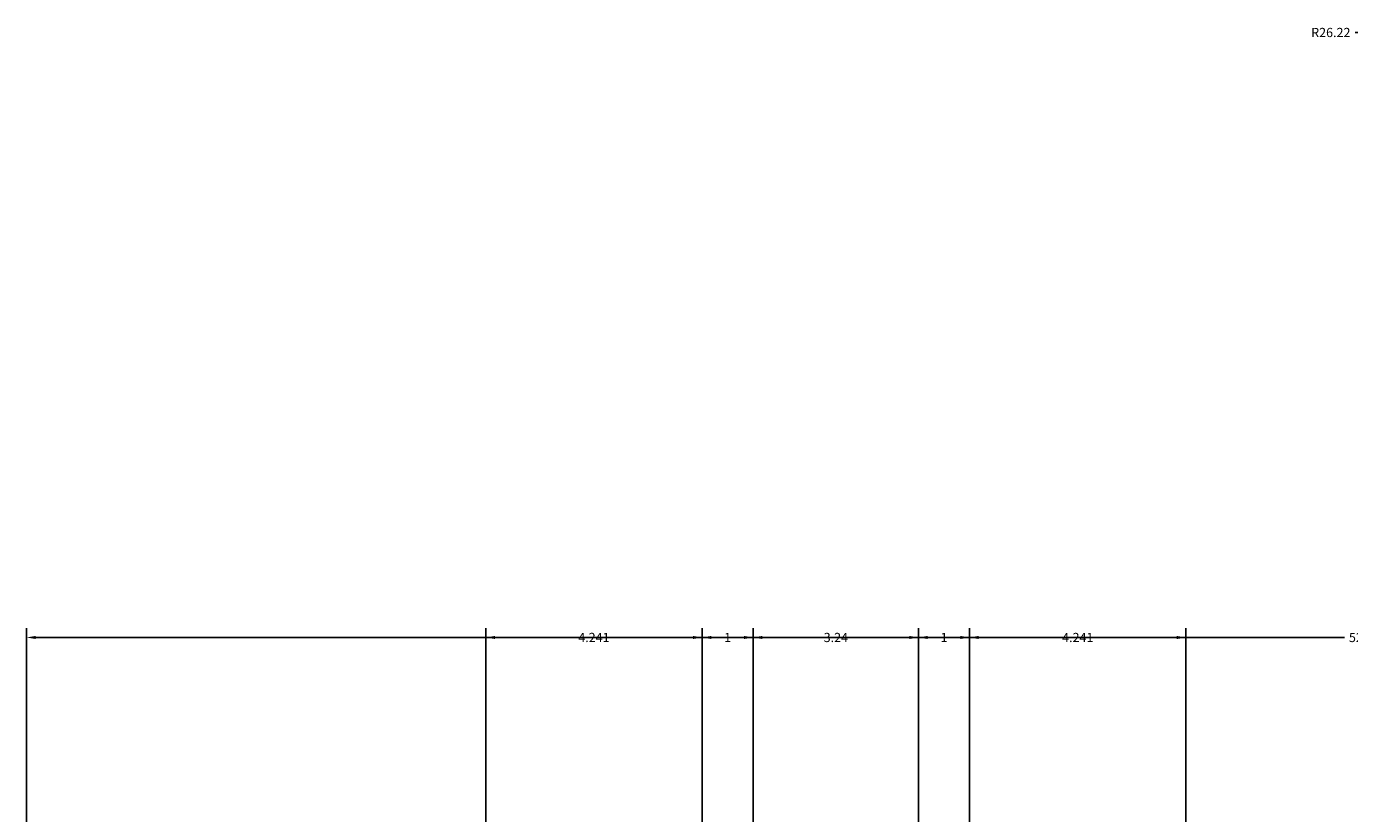
# Model space of a CAD drawing. Units: inches. Extents: x 12532.3 to 12594.9, y 6967.5 to 7063.
# Tile 7 of 9: x 12536.5 to 12562.4, y 7047.6 to 7063. Entities that reach past the tile are written whole.
import ezdxf

# ---------------------------------------------------------------- set-up
doc = ezdxf.new("R2010")
doc.units = ezdxf.units.IN
doc.header["$MEASUREMENT"] = 0
doc.header["$PDMODE"] = 98
doc.layers.add('A-ANNO-DIMS', color=2, linetype='Continuous', lineweight=18)
doc.styles.get("Standard").update_dxf_attribs({"font": 'arial.ttf'})
doc.dimstyles.get("Standard").update_dxf_attribs({"dimtxt": 0.18, "dimasz": 0.18, "dimexe": 0.18, "dimexo": 0.0625, "dimgap": 0.09, "dimtad": 0, "dimtih": 1, "dimtoh": 1, "dimdec": 4, "dimzin": 0, "dimdsep": 46, "dimtxsty": 'Standard', "dimcen": 0.09, "dimadec": 0, "dimazin": 0, "dimtfac": 1, "dimtdec": 4, "dimtofl": 0, "dimtmove": 0, "dimatfit": 3, "dimfxl": 1, "dimtolj": 1, "dimtzin": 0, "dimarcsym": 0})

# ---------------------------------------------------------------- blocks, each defined once
blk = doc.blocks.new('*D31')
at = {"layer": 'A-ANNO-DIMS', "color": 0, "lineweight": -2, "transparency": 16777216}
for p, q in [((12536.45, 7020.991), (12536.45, 7051.211)), ((12588.894, 7020.991), (12588.894, 7051.211)), ((12536.63, 7051.031), (12562.279, 7051.031)), ((12588.714, 7051.031), (12563.065, 7051.031))]:
    blk.add_line(p, q, dxfattribs=at)
at = {"layer": 'A-ANNO-DIMS', "color": 0, "transparency": 16777216}
for points in [[(12536.63, 7051.061), (12536.63, 7051.001), (12536.45, 7051.031)], [(12588.714, 7051.061), (12588.714, 7051.001), (12588.894, 7051.031)]]:
    blk.add_solid(points, dxfattribs=at)
at = {"layer": 'Defpoints', "color": 0, "transparency": 16777216}
for p in [(12588.894, 7051.031), (12536.45, 7020.929), (12588.894, 7020.929)]:
    blk.add_point(p, dxfattribs=at)
at = {"layer": 'A-ANNO-DIMS', "color": 0, "transparency": 16777216, "insert": (12562.672, 7051.031), "char_height": 0.18, "attachment_point": 5}
blk.add_mtext('\\A1;52.44', dxfattribs=at)
blk = doc.blocks.new('*D46')
at = {"layer": 'A-ANNO-DIMS', "color": 0, "lineweight": -2, "transparency": 16777216}
for p, q in [((12545.45, 7015.991), (12545.45, 7051.211)), ((12549.691, 7015.991), (12549.691, 7051.211)), ((12545.63, 7051.031), (12547.191, 7051.031)), ((12549.511, 7051.031), (12547.95, 7051.031))]:
    blk.add_line(p, q, dxfattribs=at)
at = {"layer": 'A-ANNO-DIMS', "color": 0, "transparency": 16777216}
for points in [[(12545.63, 7051.061), (12545.63, 7051.001), (12545.45, 7051.031)], [(12549.511, 7051.061), (12549.511, 7051.001), (12549.691, 7051.031)]]:
    blk.add_solid(points, dxfattribs=at)
at = {"layer": 'Defpoints', "color": 0, "transparency": 16777216}
for p in [(12549.691, 7051.031), (12545.45, 7015.929), (12549.691, 7015.929)]:
    blk.add_point(p, dxfattribs=at)
at = {"layer": 'A-ANNO-DIMS', "color": 0, "transparency": 16777216, "insert": (12547.57, 7051.031), "char_height": 0.18, "attachment_point": 5}
blk.add_mtext('\\A1;4.241', dxfattribs=at)
blk = doc.blocks.new('*D47')
at = {"layer": 'A-ANNO-DIMS', "color": 0, "lineweight": -2, "transparency": 16777216}
for p, q in [((12549.691, 7015.991), (12549.691, 7051.211)), ((12550.691, 7015.991), (12550.691, 7051.211)), ((12549.871, 7051.031), (12550.068, 7051.031)), ((12550.511, 7051.031), (12550.314, 7051.031))]:
    blk.add_line(p, q, dxfattribs=at)
at = {"layer": 'A-ANNO-DIMS', "color": 0, "transparency": 16777216}
for points in [[(12549.871, 7051.061), (12549.871, 7051.001), (12549.691, 7051.031)], [(12550.511, 7051.061), (12550.511, 7051.001), (12550.691, 7051.031)]]:
    blk.add_solid(points, dxfattribs=at)
at = {"layer": 'Defpoints', "color": 0, "transparency": 16777216}
for p in [(12550.691, 7051.031), (12549.691, 7015.929), (12550.691, 7015.929)]:
    blk.add_point(p, dxfattribs=at)
at = {"layer": 'A-ANNO-DIMS', "color": 0, "transparency": 16777216, "insert": (12550.191, 7051.031), "char_height": 0.18, "attachment_point": 5}
blk.add_mtext('\\A1;1', dxfattribs=at)
blk = doc.blocks.new('*D48')
at = {"layer": 'A-ANNO-DIMS', "color": 0, "lineweight": -2, "transparency": 16777216}
for p, q in [((12550.691, 7015.991), (12550.691, 7051.211)), ((12553.931, 7015.991), (12553.931, 7051.211)), ((12550.871, 7051.031), (12551.988, 7051.031)), ((12553.751, 7051.031), (12552.634, 7051.031))]:
    blk.add_line(p, q, dxfattribs=at)
at = {"layer": 'A-ANNO-DIMS', "color": 0, "transparency": 16777216}
for points in [[(12550.871, 7051.061), (12550.871, 7051.001), (12550.691, 7051.031)], [(12553.751, 7051.061), (12553.751, 7051.001), (12553.931, 7051.031)]]:
    blk.add_solid(points, dxfattribs=at)
at = {"layer": 'Defpoints', "color": 0, "transparency": 16777216}
for p in [(12553.931, 7051.031), (12550.691, 7015.929), (12553.931, 7015.929)]:
    blk.add_point(p, dxfattribs=at)
at = {"layer": 'A-ANNO-DIMS', "color": 0, "transparency": 16777216, "insert": (12552.311, 7051.031), "char_height": 0.18, "attachment_point": 5}
blk.add_mtext('\\A1;3.24', dxfattribs=at)
blk = doc.blocks.new('*D49')
at = {"layer": 'A-ANNO-DIMS', "color": 0, "lineweight": -2, "transparency": 16777216}
for p, q in [((12553.931, 7015.991), (12553.931, 7051.211)), ((12554.931, 7015.991), (12554.931, 7051.211)), ((12554.111, 7051.031), (12554.308, 7051.031)), ((12554.751, 7051.031), (12554.555, 7051.031))]:
    blk.add_line(p, q, dxfattribs=at)
at = {"layer": 'A-ANNO-DIMS', "color": 0, "transparency": 16777216}
for points in [[(12554.111, 7051.061), (12554.111, 7051.001), (12553.931, 7051.031)], [(12554.751, 7051.061), (12554.751, 7051.001), (12554.931, 7051.031)]]:
    blk.add_solid(points, dxfattribs=at)
at = {"layer": 'Defpoints', "color": 0, "transparency": 16777216}
for p in [(12554.931, 7051.031), (12553.931, 7015.929), (12554.931, 7015.929)]:
    blk.add_point(p, dxfattribs=at)
at = {"layer": 'A-ANNO-DIMS', "color": 0, "transparency": 16777216, "insert": (12554.431, 7051.031), "char_height": 0.18, "attachment_point": 5}
blk.add_mtext('\\A1;1', dxfattribs=at)
blk = doc.blocks.new('*D50')
at = {"layer": 'A-ANNO-DIMS', "color": 0, "lineweight": -2, "transparency": 16777216}
for p, q in [((12554.931, 7015.991), (12554.931, 7051.211)), ((12559.172, 7015.991), (12559.172, 7051.211)), ((12555.111, 7051.031), (12556.672, 7051.031)), ((12558.992, 7051.031), (12557.432, 7051.031))]:
    blk.add_line(p, q, dxfattribs=at)
at = {"layer": 'A-ANNO-DIMS', "color": 0, "transparency": 16777216}
for points in [[(12555.111, 7051.061), (12555.111, 7051.001), (12554.931, 7051.031)], [(12558.992, 7051.061), (12558.992, 7051.001), (12559.172, 7051.031)]]:
    blk.add_solid(points, dxfattribs=at)
at = {"layer": 'Defpoints', "color": 0, "transparency": 16777216}
for p in [(12559.172, 7051.031), (12554.931, 7015.929), (12559.172, 7015.929)]:
    blk.add_point(p, dxfattribs=at)
at = {"layer": 'A-ANNO-DIMS', "color": 0, "transparency": 16777216, "insert": (12557.052, 7051.031), "char_height": 0.18, "attachment_point": 5}
blk.add_mtext('\\A1;4.241', dxfattribs=at)
blk = doc.blocks.new('*D62')
at = {"layer": 'A-ANNO-DIMS', "color": 0, "lineweight": -2, "transparency": 16777216}
for p, q in [((12562.489, 7062.884), (12562.669, 7062.884)), ((12562.669, 7062.884), (12562.67, 7047.331)), ((12562.672, 7020.839), (12562.672, 7021.019)), ((12562.582, 7020.929), (12562.762, 7020.929))]:
    blk.add_line(p, q, dxfattribs=at)
at = {"layer": 'A-ANNO-DIMS', "color": 0, "transparency": 16777216}
blk.add_solid([(12562.7, 7047.331), (12562.64, 7047.331), (12562.67, 7047.151)], dxfattribs=at)
at = {"layer": 'Defpoints', "color": 0, "transparency": 16777216}
for p in [(12562.67, 7047.151), (12562.672, 7020.929)]:
    blk.add_point(p, dxfattribs=at)
at = {"layer": 'A-ANNO-DIMS', "color": 0, "transparency": 16777216, "insert": (12562.01, 7062.884), "char_height": 0.18, "attachment_point": 5}
blk.add_mtext('\\A1;R26.22', dxfattribs=at)

msp = doc.modelspace()

# ---------------------------------------------------------------- dimensions: what is measured, and where the dimension line sits
at = {"layer": 'A-ANNO-DIMS'}
dim = msp.add_radius_dim(center=(12562.6721, 7020.9287), mpoint=(12562.67, 7047.1506), dimstyle='Standard', override={"dimdec": 2, "dimlfac": 1, "dimrnd": 0, "dimzin": 0, "dimdsep": 46, "dimlunit": 2}, dxfattribs=at)
dim.commit()
dim.dimension.update_dxf_attribs({"geometry": '*D62', "text_midpoint": (12562.0098, 7062.8838), "dimtype": 164})
for base, p1, p2, override, picture, middle in [((12588.894, 7051.0306), (12536.4501, 7020.9287), (12588.894, 7020.9287), {"dimdec": 2, "dimlfac": 1, "dimrnd": 0, "dimzin": 0, "dimdsep": 46, "dimlunit": 2}, '*D31', (12562.6721, 7051.0306)), ((12549.6908, 7051.0306), (12545.4501, 7015.9287), (12549.6908, 7015.9287), {"dimdec": 3, "dimlfac": 1, "dimrnd": 0, "dimzin": 0, "dimdsep": 46, "dimlunit": 2}, '*D46', (12547.5705, 7051.0306)), ((12550.6908, 7051.0306), (12549.6908, 7015.9287), (12550.6908, 7015.9287), {"dimdec": 0, "dimlfac": 1, "dimrnd": 0, "dimzin": 0, "dimdsep": 46, "dimlunit": 2}, '*D47', (12550.1908, 7051.0306)), ((12553.9314, 7051.0306), (12550.6908, 7015.9287), (12553.9314, 7015.9287), {"dimdec": 2, "dimlfac": 1, "dimrnd": 0, "dimzin": 0, "dimdsep": 46, "dimlunit": 2}, '*D48', (12552.3111, 7051.0306)), ((12554.9314, 7051.0306), (12553.9314, 7015.9287), (12554.9314, 7015.9287), {"dimdec": 0, "dimlfac": 1, "dimrnd": 0, "dimzin": 0, "dimdsep": 46, "dimlunit": 2}, '*D49', (12554.4314, 7051.0306)), ((12559.1721, 7051.0306), (12554.9314, 7015.9287), (12559.1721, 7015.9287), {"dimdec": 3, "dimlfac": 1, "dimrnd": 0, "dimzin": 0, "dimdsep": 46, "dimlunit": 2}, '*D50', (12557.0518, 7051.0306))]:
    dim = msp.add_linear_dim(base=base, p1=p1, p2=p2, dimstyle='Standard', override=override, dxfattribs=at)
    dim.commit()
    dim.dimension.update_dxf_attribs({"geometry": picture, "text_midpoint": middle})

doc.saveas('drawing.dxf')
